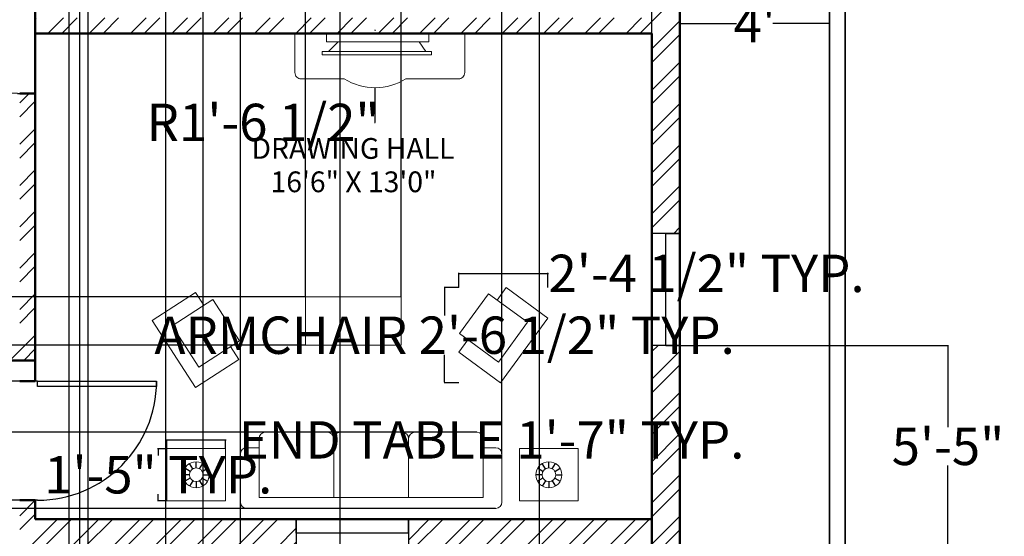
# Model space of a CAD drawing. Units: inches. Extents: x -40 to 578, y -482 to 237.
# Tile 3 of 7: x 219 to 535, y -295 to -129. Entities that reach past the tile are written whole.
import ezdxf

# ---------------------------------------------------------------- set-up
doc = ezdxf.new("R2010")
doc.units = ezdxf.units.IN
doc.header["$MEASUREMENT"] = 0
for name, color, linetype, lineweight in [('A-ANNO-DIMS', 2, 'Continuous', 18), ('A-AREA-IDEN', 240, 'Continuous', 25), ('A-FURN', 4, 'Continuous', 18), ('A-WALL-PATT', 252, 'Continuous', 13), ('C-PROP', 3, 'Continuous', 35), ('DOORS', 2, 'Continuous', 25), ('WALLS', 3, 'Continuous', 50), ('WINDOWS', 241, 'Continuous', 25)]:
    doc.layers.add(name, color=color, linetype=linetype, lineweight=lineweight)
doc.layers.add('FURITURE', color=4, linetype='Continuous')
doc.styles.get("Standard").update_dxf_attribs({"font": 'arial.ttf'})
doc.dimstyles.get("Standard").update_dxf_attribs({"dimtxt": 12, "dimasz": 0.18, "dimexe": 0.18, "dimexo": 0.0625, "dimgap": 0.09, "dimtad": 0, "dimtih": 1, "dimtoh": 1, "dimdec": 0, "dimzin": 0, "dimdsep": 46, "dimlunit": 3, "dimtxsty": 'Standard', "dimcen": 0.09, "dimadec": 0, "dimazin": 0, "dimtfac": 1, "dimtdec": 0, "dimtofl": 0, "dimtmove": 0, "dimatfit": 3, "dimfxl": 1, "dimtolj": 1, "dimtzin": 0, "dimarcsym": 0})

# ---------------------------------------------------------------- blocks, each defined once
blk = doc.blocks.new('*U10')
for p, q in [((0, 0), (0, -6)), ((40, 0), (40, -6))]:
    blk.add_line(p, q)
blk.add_lwpolyline([(0, 0), (0, 40), (1.75, 40), (1.75, 0)], close=True)
blk.add_arc((0, 0), 40, 0, 90)
blk = doc.blocks.new('*D19')
at = {"layer": 'A-ANNO-DIMS', "color": 0, "lineweight": -2, "transparency": 16777216}
for p, q in [((430.74, -125.2), (430.74, -130.58)), ((478.74, -125.2), (478.74, -130.58)), ((430.92, -130.4), (448.89, -130.4)), ((478.56, -130.4), (460.59, -130.4))]:
    blk.add_line(p, q, dxfattribs=at)
at = {"layer": 'A-ANNO-DIMS', "color": 0, "transparency": 16777216}
for points in [[(430.92, -130.37), (430.92, -130.43), (430.74, -130.4)], [(478.56, -130.37), (478.56, -130.43), (478.74, -130.4)]]:
    blk.add_solid(points, dxfattribs=at)
at = {"layer": 'Defpoints', "color": 0, "transparency": 16777216}
for p in [(430.74, -125.13), (478.74, -125.13), (478.74, -130.4)]:
    blk.add_point(p, dxfattribs=at)
at = {"layer": 'A-ANNO-DIMS', "color": 0, "transparency": 16777216, "insert": (454.74, -130.4), "char_height": 12, "attachment_point": 5}
blk.add_mtext("\\A1;4'", dxfattribs=at)
blk = doc.blocks.new('WIN-36IN')
for p, q in [((9, 36), (0, 36)), ((4.5, 0), (4.5, 36)), ((4.5, 36), (9, 36)), ((9, 0), (0, 0)), ((4.5, 0), (9, 0))]:
    blk.add_line(p, q)
blk = doc.blocks.new('CHAIR-LOUNGE')
for p, q in [((12.29, 26.57), (15.2, 30.54)), ((15.2, 30.54), (28.59, 20.71)), ((28.59, 20.71), (13.39, 0)), ((2.91, 13.79), (0, 9.83)), ((0, 9.83), (13.39, 0))]:
    blk.add_line(p, q)
blk.add_lwpolyline([(0.15, 15.82), (9.53, 28.6), (22.05, 19.41), (12.67, 6.63)], close=True)
blk = doc.blocks.new('*U3')
at = {"layer": 'FURITURE'}
blk.add_line((0, -1), (0, 1), dxfattribs=at)
blk = doc.blocks.new('*U4')
at = {"layer": 'FURITURE', "transparency": 16777216}
blk.add_blockref('*U3', (256.95, -272.5), dxfattribs=at)
for p, rotation in [((254.19, -274.1), 59.99999999999999), ((255.35, -272.93), 29.99999999999998), ((258.54, -272.93), 329.9999999999999), ((259.71, -274.1), 300), ((253.76, -275.69), 90), ((254.19, -277.28), 120), ((255.35, -278.45), 150), ((256.95, -278.88), 180), ((258.54, -278.45), 210), ((259.71, -277.28), 240), ((260.13, -275.69), 270)]:
    blk.add_blockref('*U3', p, dxfattribs=dict(at, rotation=rotation))
blk = doc.blocks.new('END-TABLE-LAMP')
blk.add_lwpolyline([(18.78, 0), (0, 0), (0, 16.79), (18.78, 16.79)], close=True)
for radius in [4.19, 2.19]:
    blk.add_circle((9.39, 8.39), radius)
blk.add_blockref('*U4', (-247.56, 284.08))
blk = doc.blocks.new('*D36')
at = {"layer": 'A-ANNO-DIMS', "color": 0, "lineweight": -2, "transparency": 16777216}
for p, q in [((359.69, -215.19), (354.99, -215.19)), ((355.17, -215.37), (355.17, -224.17)), ((355.17, -245.55), (355.17, -236.76)), ((359.69, -245.73), (354.99, -245.73))]:
    blk.add_line(p, q, dxfattribs=at)
at = {"layer": 'A-ANNO-DIMS', "color": 0, "transparency": 16777216}
for points in [[(355.14, -215.37), (355.2, -215.37), (355.17, -215.19)], [(355.14, -245.55), (355.2, -245.55), (355.17, -245.73)]]:
    blk.add_solid(points, dxfattribs=at)
at = {"layer": 'Defpoints', "color": 0, "transparency": 16777216}
for p in [(355.17, -215.19), (359.75, -215.19), (359.75, -245.73)]:
    blk.add_point(p, dxfattribs=at)
at = {"layer": 'A-ANNO-DIMS', "color": 0, "transparency": 16777216, "insert": (355.17, -230.46), "char_height": 12, "attachment_point": 5}
blk.add_mtext('\\A1;ARMCHAIR 2\'-6 1/2" TYP.', dxfattribs=at)
blk = doc.blocks.new('*D37')
at = {"layer": 'A-ANNO-DIMS', "color": 0, "lineweight": -2, "transparency": 16777216}
for p, q in [((359.75, -215.13), (359.75, -210.43)), ((359.93, -210.61), (388.16, -210.61)), ((388.34, -215.13), (388.34, -210.43)), ((388.34, -210.61), (388.52, -210.61))]:
    blk.add_line(p, q, dxfattribs=at)
at = {"layer": 'A-ANNO-DIMS', "color": 0, "transparency": 16777216}
for points in [[(359.93, -210.58), (359.93, -210.64), (359.75, -210.61)], [(388.16, -210.58), (388.16, -210.64), (388.34, -210.61)]]:
    blk.add_solid(points, dxfattribs=at)
at = {"layer": 'Defpoints', "color": 0, "transparency": 16777216}
for p in [(388.34, -210.61), (359.75, -215.19), (388.34, -215.19)]:
    blk.add_point(p, dxfattribs=at)
at = {"layer": 'A-ANNO-DIMS', "color": 0, "transparency": 16777216, "insert": (439.27, -210.61), "char_height": 12, "attachment_point": 5}
blk.add_mtext('\\A1;2\'-4 1/2" TYP.', dxfattribs=at)
blk = doc.blocks.new('*D38')
at = {"layer": 'A-ANNO-DIMS', "color": 0, "lineweight": -2, "transparency": 16777216}
for p, q in [((266.02, -266.84), (266.02, -263.91)), ((266.2, -264.09), (284.63, -264.09)), ((284.81, -266.84), (284.81, -263.91)), ((284.81, -264.09), (284.99, -264.09))]:
    blk.add_line(p, q, dxfattribs=at)
at = {"layer": 'A-ANNO-DIMS', "color": 0, "transparency": 16777216}
for points in [[(266.2, -264.06), (266.2, -264.12), (266.02, -264.09)], [(284.63, -264.06), (284.63, -264.12), (284.81, -264.09)]]:
    blk.add_solid(points, dxfattribs=at)
at = {"layer": 'Defpoints', "color": 0, "transparency": 16777216}
for p in [(284.81, -264.09), (266.02, -266.91), (284.81, -266.91)]:
    blk.add_point(p, dxfattribs=at)
at = {"layer": 'A-ANNO-DIMS', "color": 0, "transparency": 16777216, "insert": (370.24, -264.09), "char_height": 12, "attachment_point": 5}
blk.add_mtext('\\A1;END TABLE 1\'-7" TYP.', dxfattribs=at)
blk = doc.blocks.new('*D39')
at = {"layer": 'A-ANNO-DIMS', "color": 0, "lineweight": -2, "transparency": 16777216}
for p, q in [((265.96, -266.91), (263.03, -266.91)), ((263.21, -267.09), (263.21, -269.08)), ((265.96, -283.69), (263.03, -283.69)), ((263.21, -283.51), (263.21, -281.52))]:
    blk.add_line(p, q, dxfattribs=at)
at = {"layer": 'A-ANNO-DIMS', "color": 0, "transparency": 16777216}
for points in [[(263.18, -267.09), (263.24, -267.09), (263.21, -266.91)], [(263.18, -283.51), (263.24, -283.51), (263.21, -283.69)]]:
    blk.add_solid(points, dxfattribs=at)
at = {"layer": 'Defpoints', "color": 0, "transparency": 16777216}
for p in [(263.21, -266.91), (266.02, -266.91), (266.02, -283.69)]:
    blk.add_point(p, dxfattribs=at)
at = {"layer": 'A-ANNO-DIMS', "color": 0, "transparency": 16777216, "insert": (263.21, -275.3), "char_height": 12, "attachment_point": 5}
blk.add_mtext('\\A1;1\'-5" TYP.', dxfattribs=at)
blk = doc.blocks.new('*D49')
at = {"layer": 'A-ANNO-DIMS', "color": 0, "lineweight": -2, "transparency": 16777216}
for p, q in [((385.66, -377.49), (385.66, 219.12)), ((385.84, 218.94), (387.66, 218.94)), ((421.56, 218.94), (419.73, 218.94)), ((421.74, -377.49), (421.74, 219.12))]:
    blk.add_line(p, q, dxfattribs=at)
at = {"layer": 'A-ANNO-DIMS', "color": 0, "transparency": 16777216}
for points in [[(385.84, 218.97), (385.84, 218.91), (385.66, 218.94)], [(421.56, 218.97), (421.56, 218.91), (421.74, 218.94)]]:
    blk.add_solid(points, dxfattribs=at)
at = {"layer": 'Defpoints', "color": 0, "transparency": 16777216}
for p in [(421.74, 218.94), (385.66, -377.55), (421.74, -377.55)]:
    blk.add_point(p, dxfattribs=at)
at = {"layer": 'A-ANNO-DIMS', "color": 0, "transparency": 16777216, "insert": (403.7, 218.94), "char_height": 12, "attachment_point": 5}
blk.add_mtext('\\A1;3\'-0"', dxfattribs=at)
blk = doc.blocks.new('*D50')
at = {"layer": 'A-ANNO-DIMS', "color": 0, "lineweight": -2, "transparency": 16777216}
for p, q in [((265.66, -330.99), (265.66, 219.12)), ((265.84, 218.94), (277.48, 218.94)), ((277.66, -330.99), (277.66, 219.12)), ((277.66, 218.94), (277.84, 218.94))]:
    blk.add_line(p, q, dxfattribs=at)
at = {"layer": 'A-ANNO-DIMS', "color": 0, "transparency": 16777216}
for points in [[(265.84, 218.97), (265.84, 218.91), (265.66, 218.94)], [(277.48, 218.97), (277.48, 218.91), (277.66, 218.94)]]:
    blk.add_solid(points, dxfattribs=at)
at = {"layer": 'Defpoints', "color": 0, "transparency": 16777216}
for p in [(277.66, 218.94), (265.66, -331.05), (277.66, -331.05)]:
    blk.add_point(p, dxfattribs=at)
at = {"layer": 'A-ANNO-DIMS', "color": 0, "transparency": 16777216, "insert": (293.31, 218.94), "char_height": 12, "attachment_point": 5}
blk.add_mtext('\\A1;1\'-0"', dxfattribs=at)
blk = doc.blocks.new('*D52')
at = {"layer": 'A-ANNO-DIMS', "color": 0, "lineweight": -2, "transparency": 16777216}
for p, q in [((234.57, -377.49), (234.57, 219.12)), ((234.75, 218.94), (265.48, 218.94)), ((265.66, -377.49), (265.66, 219.12)), ((265.66, 218.94), (265.84, 218.94))]:
    blk.add_line(p, q, dxfattribs=at)
at = {"layer": 'A-ANNO-DIMS', "color": 0, "transparency": 16777216}
for points in [[(234.75, 218.97), (234.75, 218.91), (234.57, 218.94)], [(265.48, 218.97), (265.48, 218.91), (265.66, 218.94)]]:
    blk.add_solid(points, dxfattribs=at)
at = {"layer": 'Defpoints', "color": 0, "transparency": 16777216}
for p in [(265.66, 218.94), (234.57, -377.55), (265.66, -377.55)]:
    blk.add_point(p, dxfattribs=at)
at = {"layer": 'A-ANNO-DIMS', "color": 0, "transparency": 16777216, "insert": (281.98, 218.94), "char_height": 12, "attachment_point": 5}
blk.add_mtext('\\A1;2\'-7"', dxfattribs=at)
blk = doc.blocks.new('*D54')
at = {"layer": 'A-ANNO-DIMS', "color": 0, "lineweight": -2, "transparency": 16777216}
for p, q in [((202.4, 25.39), (202.4, -474.78)), ((240.62, 25.39), (240.62, -474.78)), ((202.58, -474.6), (205.48, -474.6)), ((240.44, -474.6), (237.55, -474.6))]:
    blk.add_line(p, q, dxfattribs=at)
at = {"layer": 'A-ANNO-DIMS', "color": 0, "transparency": 16777216}
for points in [[(202.58, -474.57), (202.58, -474.63), (202.4, -474.6)], [(240.44, -474.57), (240.44, -474.63), (240.62, -474.6)]]:
    blk.add_solid(points, dxfattribs=at)
at = {"layer": 'Defpoints', "color": 0, "transparency": 16777216}
for p in [(202.4, 25.45), (240.62, 25.45), (240.62, -474.6)]:
    blk.add_point(p, dxfattribs=at)
at = {"layer": 'A-ANNO-DIMS', "color": 0, "transparency": 16777216, "insert": (221.51, -474.6), "char_height": 12, "attachment_point": 5}
blk.add_mtext('\\A1;3\'-2"', dxfattribs=at)
blk = doc.blocks.new('*D60')
at = {"layer": 'A-ANNO-DIMS', "color": 0, "lineweight": -2, "transparency": 16777216}
for p, q in [((218.68, -245.25), (-3.49, -245.25)), ((-3.31, -245.43), (-3.31, -258.14)), ((-3.31, -283.29), (-3.31, -270.58)), ((218.68, -283.47), (-3.49, -283.47))]:
    blk.add_line(p, q, dxfattribs=at)
at = {"layer": 'A-ANNO-DIMS', "color": 0, "transparency": 16777216}
for points in [[(-3.34, -245.43), (-3.28, -245.43), (-3.31, -245.25)], [(-3.34, -283.29), (-3.28, -283.29), (-3.31, -283.47)]]:
    blk.add_solid(points, dxfattribs=at)
at = {"layer": 'Defpoints', "color": 0, "transparency": 16777216}
for p in [(-3.31, -245.25), (218.74, -245.25), (218.74, -283.47)]:
    blk.add_point(p, dxfattribs=at)
at = {"layer": 'A-ANNO-DIMS', "color": 0, "transparency": 16777216, "insert": (-3.31, -264.36), "char_height": 12, "attachment_point": 5}
blk.add_mtext('\\A1;3\'-2"', dxfattribs=at)
blk = doc.blocks.new('*D69')
at = {"layer": 'A-ANNO-DIMS', "color": 0, "lineweight": -2, "transparency": 16777216}
for p, q in [((321.5, -125.98), (321.5, -474.78)), ((289.56, -128.61), (289.56, -474.78)), ((289.74, -474.6), (321.32, -474.6)), ((321.5, -474.6), (321.68, -474.6))]:
    blk.add_line(p, q, dxfattribs=at)
at = {"layer": 'A-ANNO-DIMS', "color": 0, "transparency": 16777216}
for points in [[(289.74, -474.57), (289.74, -474.63), (289.56, -474.6)], [(321.32, -474.57), (321.32, -474.63), (321.5, -474.6)]]:
    blk.add_solid(points, dxfattribs=at)
at = {"layer": 'Defpoints', "color": 0, "transparency": 16777216}
for p in [(321.5, -125.92), (289.56, -128.55), (321.5, -474.6)]:
    blk.add_point(p, dxfattribs=at)
at = {"layer": 'A-ANNO-DIMS', "color": 0, "transparency": 16777216, "insert": (337.82, -474.6), "char_height": 12, "attachment_point": 5}
blk.add_mtext('\\A1;2\'-8"', dxfattribs=at)
blk = doc.blocks.new('*D71')
at = {"layer": 'A-ANNO-DIMS', "color": 0, "lineweight": -2, "transparency": 16777216}
for p, q in [((184.88, -63.19), (184.88, -474.78)), ((237.97, -63.19), (237.97, -474.78)), ((185.06, -474.6), (195.15, -474.6)), ((237.79, -474.6), (227.71, -474.6))]:
    blk.add_line(p, q, dxfattribs=at)
at = {"layer": 'A-ANNO-DIMS', "color": 0, "transparency": 16777216}
for points in [[(185.06, -474.57), (185.06, -474.63), (184.88, -474.6)], [(237.79, -474.57), (237.79, -474.63), (237.97, -474.6)]]:
    blk.add_solid(points, dxfattribs=at)
at = {"layer": 'Defpoints', "color": 0, "transparency": 16777216}
for p in [(184.88, -63.12), (237.97, -63.12), (237.97, -474.6)]:
    blk.add_point(p, dxfattribs=at)
at = {"layer": 'A-ANNO-DIMS', "color": 0, "transparency": 16777216, "insert": (211.43, -474.6), "char_height": 12, "attachment_point": 5}
blk.add_mtext('\\A1;4\'-5"', dxfattribs=at)
blk = doc.blocks.new('*D73')
at = {"layer": 'A-ANNO-DIMS', "color": 0, "lineweight": -2, "transparency": 16777216}
for p, q in [((289.59, -268.55), (289.59, 219.12)), ((289.77, 218.94), (315.6, 218.94)), ((373.41, 218.94), (347.58, 218.94)), ((373.59, -268.55), (373.59, 219.12))]:
    blk.add_line(p, q, dxfattribs=at)
at = {"layer": 'A-ANNO-DIMS', "color": 0, "transparency": 16777216}
for points in [[(289.77, 218.97), (289.77, 218.91), (289.59, 218.94)], [(373.41, 218.97), (373.41, 218.91), (373.59, 218.94)]]:
    blk.add_solid(points, dxfattribs=at)
at = {"layer": 'Defpoints', "color": 0, "transparency": 16777216}
for p in [(373.59, 218.94), (289.59, -268.61), (373.59, -268.61)]:
    blk.add_point(p, dxfattribs=at)
at = {"layer": 'A-ANNO-DIMS', "color": 0, "transparency": 16777216, "insert": (331.59, 218.94), "char_height": 12, "attachment_point": 5}
blk.add_mtext('\\A1;7\'-0"', dxfattribs=at)
blk = doc.blocks.new('*D74')
at = {"layer": 'A-ANNO-DIMS', "color": 0, "lineweight": -2, "transparency": 16777216}
for p, q in [((365.53, -261.64), (-3.49, -261.64)), ((-3.31, -261.82), (-3.31, -267.57)), ((-3.31, -285.9), (-3.31, -280.16)), ((371.53, -286.08), (-3.49, -286.08))]:
    blk.add_line(p, q, dxfattribs=at)
at = {"layer": 'A-ANNO-DIMS', "color": 0, "transparency": 16777216}
for points in [[(-3.34, -261.82), (-3.28, -261.82), (-3.31, -261.64)], [(-3.34, -285.9), (-3.28, -285.9), (-3.31, -286.08)]]:
    blk.add_solid(points, dxfattribs=at)
at = {"layer": 'Defpoints', "color": 0, "transparency": 16777216}
for p in [(365.59, -261.64), (-3.31, -286.08), (371.59, -286.08)]:
    blk.add_point(p, dxfattribs=at)
at = {"layer": 'A-ANNO-DIMS', "color": 0, "transparency": 16777216, "insert": (-3.31, -273.86), "char_height": 12, "attachment_point": 5}
blk.add_mtext('\\A1;2\'-0 1/2"', dxfattribs=at)
blk = doc.blocks.new('*D75')
at = {"layer": 'A-ANNO-DIMS', "color": 0, "lineweight": -2, "transparency": 16777216}
for p, q in [((310.54, -218.11), (310.54, 219.12)), ((310.72, 218.94), (340.99, 218.94)), ((341.17, -218.11), (341.17, 219.12)), ((341.17, 218.94), (341.35, 218.94))]:
    blk.add_line(p, q, dxfattribs=at)
at = {"layer": 'A-ANNO-DIMS', "color": 0, "transparency": 16777216}
for points in [[(310.72, 218.97), (310.72, 218.91), (310.54, 218.94)], [(340.99, 218.97), (340.99, 218.91), (341.17, 218.94)]]:
    blk.add_solid(points, dxfattribs=at)
at = {"layer": 'Defpoints', "color": 0, "transparency": 16777216}
for p in [(341.17, 218.94), (310.54, -218.17), (341.17, -218.17)]:
    blk.add_point(p, dxfattribs=at)
at = {"layer": 'A-ANNO-DIMS', "color": 0, "transparency": 16777216, "insert": (371.48, 218.94), "char_height": 12, "attachment_point": 5}
blk.add_mtext('\\A1;2\'-6 1/2"', dxfattribs=at)
blk = doc.blocks.new('*D76')
at = {"layer": 'A-ANNO-DIMS', "color": 0, "lineweight": -2, "transparency": 16777216}
for p, q in [((310.48, -218.17), (-3.49, -218.17)), ((-3.31, -218.35), (-3.31, -219.63)), ((310.48, -233.69), (-3.49, -233.69)), ((-3.31, -233.51), (-3.31, -232.23))]:
    blk.add_line(p, q, dxfattribs=at)
at = {"layer": 'A-ANNO-DIMS', "color": 0, "transparency": 16777216}
for points in [[(-3.34, -218.35), (-3.28, -218.35), (-3.31, -218.17)], [(-3.34, -233.51), (-3.28, -233.51), (-3.31, -233.69)]]:
    blk.add_solid(points, dxfattribs=at)
at = {"layer": 'Defpoints', "color": 0, "transparency": 16777216}
for p in [(310.54, -218.17), (-3.31, -233.69), (310.54, -233.69)]:
    blk.add_point(p, dxfattribs=at)
at = {"layer": 'A-ANNO-DIMS', "color": 0, "transparency": 16777216, "insert": (-3.31, -225.93), "char_height": 12, "attachment_point": 5}
blk.add_mtext('\\A1;1\'-3 1/2"', dxfattribs=at)
blk = doc.blocks.new('*D78')
at = {"layer": 'A-ANNO-DIMS', "color": 0, "lineweight": -2, "transparency": 16777216}
for p, q in [((430.8, -233.77), (516.97, -233.77)), ((516.79, -233.95), (516.79, -259.97)), ((516.79, -298.37), (516.79, -272.35)), ((421.8, -298.55), (516.97, -298.55))]:
    blk.add_line(p, q, dxfattribs=at)
at = {"layer": 'A-ANNO-DIMS', "color": 0, "transparency": 16777216}
for points in [[(516.76, -233.95), (516.82, -233.95), (516.79, -233.77)], [(516.76, -298.37), (516.82, -298.37), (516.79, -298.55)]]:
    blk.add_solid(points, dxfattribs=at)
at = {"layer": 'Defpoints', "color": 0, "transparency": 16777216}
for p in [(430.74, -233.77), (421.74, -298.55), (516.79, -298.55)]:
    blk.add_point(p, dxfattribs=at)
at = {"layer": 'A-ANNO-DIMS', "color": 0, "transparency": 16777216, "insert": (516.79, -266.16), "char_height": 12, "attachment_point": 5}
blk.add_mtext('\\A1;5\'-5"', dxfattribs=at)
blk = doc.blocks.new('*D81')
at = {"layer": 'A-ANNO-DIMS', "color": 0, "lineweight": -2, "transparency": 16777216}
for p, q in [((332.75, -132.46), (332.93, -132.46)), ((332.84, -132.55), (332.84, -132.37)), ((332.84, -162.13), (332.84, -151.18)), ((332.66, -162.13), (332.84, -162.13))]:
    blk.add_line(p, q, dxfattribs=at)
at = {"layer": 'A-ANNO-DIMS', "color": 0, "transparency": 16777216}
blk.add_solid([(332.81, -151.18), (332.87, -151.18), (332.84, -151)], dxfattribs=at)
at = {"layer": 'Defpoints', "color": 0, "transparency": 16777216}
for p in [(332.84, -132.46), (332.84, -151)]:
    blk.add_point(p, dxfattribs=at)
at = {"layer": 'A-ANNO-DIMS', "color": 0, "transparency": 16777216, "insert": (296.9, -162.13), "char_height": 12, "attachment_point": 5}
blk.add_mtext('\\A1;R1\'-6 1/2"', dxfattribs=at)

msp = doc.modelspace()

# ---------------------------------------------------------------- hatches: boundary and pattern name
at = {"layer": 'A-WALL-PATT'}
h = msp.add_hatch(dxfattribs=at)
h.set_pattern_fill('ANSI32', color=256, scale=25)
h.set_pattern_definition([(45, (-1993.713, -1175.095), (-6.629126, 6.629126), []), (45, (-1989.294, -1175.095), (-6.629126, 6.629126), [])])
h.paths.add_polyline_path([(248.74, 172.45), (71.74, 172.45), (71.74, 114.63), (80.74, 114.63), (80.74, 163.45), (248.74, 163.45)])
h.paths.add_polyline_path([(253.74, 172.45), (248.74, 172.45), (248.74, 163.45), (253.74, 163.45)])
h.paths.add_polyline_path([(253.74, 163.45), (248.74, 163.45), (248.74, 25.45), (240.62, 25.45), (240.62, 20.45), (263.71, 20.45), (263.71, 25.45), (253.74, 25.45)])
h.paths.add_polyline_path([(483.74, 172.45), (253.74, 172.45), (253.74, 163.45), (426.74, 163.45), (474.74, 163.45), (474.74, 79.45), (465.23, 79.45), (465.23, 77.2), (441.23, 77.2), (441.23, 74.45), (483.74, 74.45)])
h.paths.add_polyline_path([(80.74, 78.63), (71.74, 78.63), (71.74, 3.32), (80.74, 3.32), (80.74, 20.45), (134.6, 20.45), (134.6, 25.45), (80.74, 25.45)])
h.paths.add_polyline_path([(202.4, 25.45), (158.53, 25.45), (158.53, 20.45), (202.4, 20.45)])
h.paths.add_polyline_path([(169.74, 20.45), (164.74, 20.45), (164.74, -39.55), (80.74, -39.55), (80.74, -20.68), (71.74, -20.68), (71.74, -61.38), (80.74, -61.38), (80.74, -44.55), (164.74, -44.55), (164.74, -104.55), (169.74, -104.55), (169.74, -44.55)])
h.paths.add_polyline_path([(135.96, -104.55), (80.74, -104.55), (80.74, -85.38), (71.74, -85.38), (71.74, -155.89), (80.74, -155.89), (80.74, -109.55), (135.96, -109.55)])
h.paths.add_polyline_path([(218.74, -104.55), (159.9, -104.55), (159.9, -109.55), (218.74, -109.55)])
h.paths.add_polyline_path([(223.74, -104.55), (218.74, -104.55), (218.74, -109.55), (223.74, -109.55)])
h.paths.add_polyline_path([(223.74, -109.55), (218.74, -109.55), (218.74, -114.58), (223.74, -114.58)])
h.paths.add_polyline_path([(430.74, -85.66), (421.74, -85.66), (421.74, -128.55), (223.74, -128.55), (223.74, -133.55), (421.74, -133.55), (421.74, -197.77), (430.74, -197.77)])
h.paths.add_polyline_path([(223.74, -152.8), (218.74, -152.8), (218.74, -229.55), (151.59, -229.55), (151.59, -238.55), (223.74, -238.55), (223.74, -229.55)])
h.paths.add_polyline_path([(115.59, -229.55), (98.23, -229.55), (80.74, -229.55), (80.74, -212.75), (80.74, -191.89), (71.74, -191.89), (71.74, -238.55), (115.59, -238.55)])
h.paths.add_polyline_path([(307.53, -289.55), (223.74, -289.55), (223.74, -283.47), (218.74, -283.47), (218.74, -298.55), (307.53, -298.55)])
h.paths.add_polyline_path([(421.74, -289.55), (343.53, -289.55), (343.53, -298.55), (421.74, -298.55)])
h.paths.add_polyline_path([(430.74, -367.34), (421.74, -367.34), (421.74, -377.55), (234.57, -377.55), (234.57, -386.55), (430.74, -386.55)])
h.paths.add_polyline_path([(430.74, -298.55), (430.74, -233.77), (421.74, -233.77), (421.74, -289.55), (421.74, -298.55), (421.74, -331.34), (430.74, -331.34)])
h.paths.add_polyline_path([(430.74, -11.67), (427.15, -11.67, -0.057068), (421.74, -11.05), (421.74, -49.66), (430.74, -49.66)])
h.paths.add_polyline_path([(430.74, 31.9), (421.74, 31.9), (421.74, 25.45), (301.93, 25.45), (301.93, 20.45), (421.74, 20.45), (421.74, 12.26), (430.74, 12.26)])
h.paths.add_polyline_path([(426.74, 134.23, -0.014739), (425.33, 134.19), (421.74, 134.19), (421.74, 74.45), (441.23, 74.45), (441.23, 77.2), (441.23, 79.45), (426.74, 79.45)], flags=17)
h.paths.add_polyline_path([(430.74, 74.45), (421.74, 74.45), (421.74, 67.9), (430.74, 67.9)])

# ---------------------------------------------------------------- linework, layer by layer
at = {"layer": 'A-FURN'}
for p, q in [((321.03, -136.26), (317.87, -139.32)), ((346.99, -136.26), (349.12, -139.32)), ((317.59, -261.64), (297.59, -261.64)), ((341.59, -261.64), (321.59, -261.64)), ((365.59, -261.64), (345.59, -261.64)), ((295.59, -263.64), (295.59, -282.61)), ((319.59, -263.64), (319.59, -282.61)), ((319.59, -263.64), (319.59, -263.64)), ((343.59, -263.64), (343.59, -282.61)), ((343.59, -263.64), (343.59, -263.64)), ((367.59, -263.64), (367.59, -282.61)), ((289.59, -284.08), (289.59, -268.61)), ((291.59, -266.61), (295.59, -266.61)), ((367.59, -266.61), (371.59, -266.61)), ((373.59, -268.61), (373.59, -284.08)), ((367.59, -282.61), (295.59, -282.61)), ((371.59, -286.08), (291.59, -286.08))]:
    msp.add_line(p, q, dxfattribs=at)
msp.add_lwpolyline([(322.95, -148.15), (309.1, -148.15, -0.414214), (307.1, -146.15), (307.1, -133.55), (361.62, -133.55), (361.62, -146.15, -0.414214), (359.62, -148.15), (342.72, -148.15)], format="xyb", dxfattribs=at)
for points in [[(317.26, -133.55), (350.08, -133.55), (350.08, -136.26), (317.26, -136.26)], [(315.89, -139.32), (350.95, -139.32), (350.95, -140.43), (315.89, -140.43)], [(341.17, -233.69), (310.54, -233.69), (310.54, -218.17), (341.17, -218.17)]]:
    msp.add_lwpolyline(points, close=True, dxfattribs=at)
for centre, radius, start, end in [((332.84, -132.46), 18.54, 237.7767, 302.2233), ((297.59, -263.64), 2, 90, 180), ((317.59, -263.64), 2, 0, 90), ((321.59, -263.64), 2, 90, 180), ((341.59, -263.64), 2, 0, 90), ((345.59, -263.64), 2, 90, 180), ((365.59, -263.64), 2, 0, 90), ((291.59, -268.61), 2, 90, 180), ((371.59, -268.61), 2, 0, 90), ((291.59, -284.08), 2, 180, 270), ((371.59, -284.08), 2, 270, 0)]:
    msp.add_arc(centre, radius, start, end, dxfattribs=at)
at = {"layer": 'C-PROP'}
for p, q in [((478.74, 74.45), (478.74, -432.55)), ((483.74, 74.45), (483.74, -441.55))]:
    msp.add_line(p, q, dxfattribs=at)
at = {"layer": 'WALLS'}
for p, q in [((430.74, 74.45), (430.74, -298.55)), ((223.74, -104.55), (223.74, -229.55)), ((223.74, -133.55), (421.74, -133.55)), ((421.74, -133.55), (421.74, -289.55)), ((223.74, -152.8), (218.74, -152.8)), ((223.74, -229.55), (223.74, -245.25)), ((223.74, -238.55), (71.74, -238.55)), ((218.74, -245.25), (223.74, -245.25)), ((218.74, -283.47), (223.74, -283.47)), ((223.74, -283.47), (223.74, -289.55)), ((223.74, -289.55), (421.74, -289.55)), ((421.74, -289.55), (421.74, -377.55))]:
    msp.add_line(p, q, dxfattribs=at)

# ---------------------------------------------------------------- block references
at = {"layer": 'A-FURN', "extrusion": (0, 0, -1), "zscale": -1, "rotation": 3.338690712319671}
msp.add_blockref('CHAIR-LOUNGE', (-288.57, -248.07), dxfattribs=at)
at = {"layer": 'A-FURN'}
for name, p in [('CHAIR-LOUNGE', (359.75, -245.73)), ('END-TABLE-LAMP', (266.02, -283.69)), ('END-TABLE-LAMP', (379.25, -283.69))]:
    msp.add_blockref(name, p, dxfattribs=at)
at = {"layer": 'DOORS', "yscale": 0.9555568703817776, "zscale": 0.9555568703817776}
for p, xscale, rotation in [((218, -114.58), -0.9555568703817776, 90), ((224.47, -245.25), 0.9555568703817776, 270)]:
    msp.add_blockref('*U10', p, dxfattribs=dict(at, xscale=xscale, rotation=rotation))
at = {"layer": 'WINDOWS'}
msp.add_blockref('WIN-36IN', (421.74, -233.77), dxfattribs=at)
at = {"layer": 'WINDOWS', "rotation": 90.0000000000001}
msp.add_blockref('WIN-36IN', (343.53, -298.55), dxfattribs=at)

# ---------------------------------------------------------------- texts
at = {"layer": 'A-AREA-IDEN'}
for s, p in [('DRAWING HALL', (293.16, -173.82)), ('   16\'6" X 13\'0"', (293.16, -184.54))]:
    msp.add_text(s, height=6.6698, dxfattribs=at).set_placement(p)

# ---------------------------------------------------------------- dimensions: what is measured, and where the dimension line sits
at = {"layer": 'A-ANNO-DIMS'}
for base, p1, p2, override, picture, middle in [((341.17, 218.94), (310.54, -218.17), (341.17, -218.17), {"dimdec": 1, "dimlfac": 1, "dimrnd": 0, "dimzin": 1, "dimdsep": 46, "dimlunit": 4, "dimfrac": 2}, '*D75', (371.48, 218.94)), ((265.66, 218.94), (234.57, -377.55), (265.66, -377.55), {"dimdec": 1, "dimlfac": 1, "dimrnd": 0, "dimzin": 1, "dimdsep": 46, "dimlunit": 4, "dimfrac": 2}, '*D52', (281.98, 218.94)), ((277.66, 218.94), (265.66, -331.05), (277.66, -331.05), {"dimdec": 1, "dimlfac": 1, "dimrnd": 0, "dimzin": 1, "dimdsep": 46, "dimlunit": 4, "dimfrac": 2}, '*D50', (293.31, 218.94)), ((373.59, 218.94), (289.59, -268.61), (373.59, -268.61), {"dimdec": 1, "dimlfac": 1, "dimrnd": 0, "dimzin": 1, "dimdsep": 46, "dimlunit": 4, "dimfrac": 2}, '*D73', (331.59, 218.94)), ((421.74, 218.94), (385.66, -377.55), (421.74, -377.55), {"dimdec": 1, "dimlfac": 1, "dimrnd": 0, "dimzin": 1, "dimdsep": 46, "dimlunit": 4, "dimfrac": 2}, '*D49', (403.7, 218.94)), ((240.62, -474.6), (202.4, 25.45), (240.62, 25.45), {"dimdec": 1, "dimlfac": 1, "dimrnd": 0, "dimzin": 1, "dimdsep": 46, "dimlunit": 4, "dimfrac": 2}, '*D54', (221.51, -474.6)), ((237.97, -474.6), (184.88, -63.12), (237.97, -63.12), {"dimdec": 1, "dimlfac": 1, "dimrnd": 0, "dimzin": 1, "dimdsep": 46, "dimlunit": 4, "dimfrac": 2}, '*D71', (211.43, -474.6)), ((478.74, -130.4), (430.74, -125.13), (478.74, -125.13), {"dimclrd": 0, "dimclre": 0, "dimclrt": 0}, '*D19', (454.74, -130.4)), ((321.5, -474.6), (289.56, -128.55), (321.5, -125.92), {"dimdec": 1, "dimlfac": 1, "dimrnd": 0, "dimzin": 1, "dimdsep": 46, "dimlunit": 4, "dimfrac": 2}, '*D69', (337.82, -474.6))]:
    dim = msp.add_linear_dim(base=base, p1=p1, p2=p2, dimstyle='Standard', override=override, dxfattribs=at)
    dim.commit()
    dim.dimension.update_dxf_attribs({"geometry": picture, "text_midpoint": middle})
dim = msp.add_radius_dim(center=(332.84, -132.46), mpoint=(332.84, -151), dimstyle='Standard', override={"dimdec": 1, "dimlfac": 1, "dimrnd": 0, "dimzin": 1, "dimdsep": 46, "dimlunit": 4, "dimfrac": 2}, dxfattribs=at)
dim.commit()
dim.dimension.update_dxf_attribs({"geometry": '*D81', "text_midpoint": (296.9, -162.13), "dimtype": 164})
for base, p1, p2, text, picture, middle in [((388.34, -210.61), (359.75, -215.19), (388.34, -215.19), '<> TYP.', '*D37', (439.27, -210.61)), ((284.81, -264.09), (266.02, -266.91), (284.81, -266.91), 'END TABLE <> TYP.', '*D38', (370.24, -264.09))]:
    dim = msp.add_linear_dim(base=base, p1=p1, p2=p2, text=text, dimstyle='Standard', override={"dimdec": 1, "dimlfac": 1, "dimrnd": 0, "dimzin": 1, "dimdsep": 46, "dimlunit": 4, "dimfrac": 2}, dxfattribs=at)
    dim.commit()
    dim.dimension.update_dxf_attribs({"geometry": picture, "text_midpoint": middle})
for base, p1, p2, text, picture, middle in [((355.17, -215.19), (359.75, -245.73), (359.75, -215.19), 'ARMCHAIR <> TYP.', '*D36', (355.17, -230.46)), ((263.21, -266.91), (266.02, -283.69), (266.02, -266.91), '<> TYP.', '*D39', (263.21, -275.3))]:
    dim = msp.add_linear_dim(base=base, p1=p1, p2=p2, angle=90, text=text, dimstyle='Standard', override={"dimdec": 1, "dimlfac": 1, "dimrnd": 0, "dimzin": 1, "dimdsep": 46, "dimlunit": 4, "dimfrac": 2}, dxfattribs=at)
    dim.commit()
    dim.dimension.update_dxf_attribs({"geometry": picture, "text_midpoint": middle})
for base, p1, p2, picture, middle in [((-3.31, -233.69), (310.54, -218.17), (310.54, -233.69), '*D76', (-3.31, -225.93)), ((516.79, -298.55), (430.74, -233.77), (421.74, -298.55), '*D78', (516.79, -266.16)), ((-3.31, -245.25), (218.74, -283.47), (218.74, -245.25), '*D60', (-3.31, -264.36)), ((-3.31, -286.08), (365.59, -261.64), (371.59, -286.08), '*D74', (-3.31, -273.86))]:
    dim = msp.add_linear_dim(base=base, p1=p1, p2=p2, angle=90, dimstyle='Standard', override={"dimdec": 1, "dimlfac": 1, "dimrnd": 0, "dimzin": 1, "dimdsep": 46, "dimlunit": 4, "dimfrac": 2}, dxfattribs=at)
    dim.commit()
    dim.dimension.update_dxf_attribs({"geometry": picture, "text_midpoint": middle})

doc.saveas('drawing.dxf')
